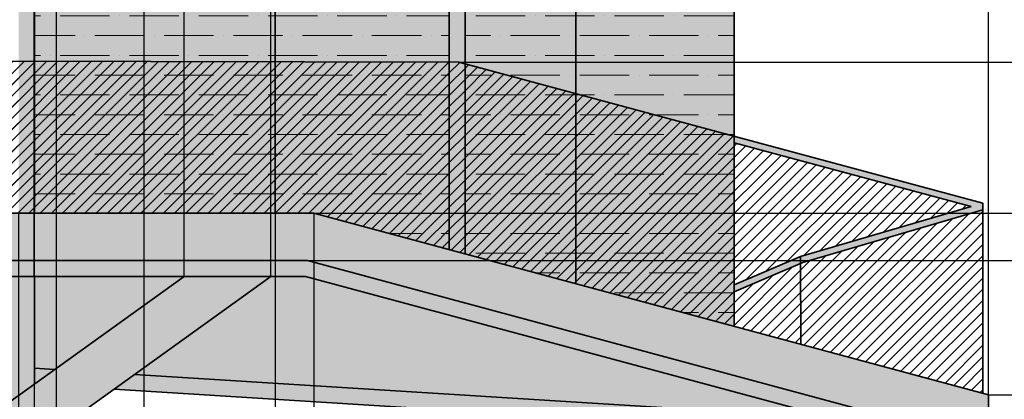
# Model space of a CAD drawing. Units: millimetres. Extents: x -504 to 6314, y 1290 to 4335.
# Tile 7 of 9: x 3796 to 5350, y 2332 to 2932. Entities that reach past the tile are written whole.
import ezdxf

# ---------------------------------------------------------------- set-up
doc = ezdxf.new("R2010")
doc.units = ezdxf.units.MM
doc.header["$MEASUREMENT"] = 0
for name, color, linetype, lineweight in [('A-ANNO-DIMS', 2, 'Continuous', 18), ('A-ELEV', 7, 'Continuous', 35), ('A-ELEV-PATT', 8, 'Continuous', 13)]:
    doc.layers.add(name, color=color, linetype=linetype, lineweight=lineweight)
doc.styles.get("Standard").update_dxf_attribs({"font": 'arial.ttf'})
doc.dimstyles.get("Standard").update_dxf_attribs({"dimtxt": 150, "dimasz": 100, "dimexe": 0.18, "dimexo": 0.0625, "dimgap": 0.09, "dimtad": 0, "dimtih": 1, "dimtoh": 1, "dimdec": 0, "dimzin": 0, "dimdsep": 46, "dimtxsty": 'Standard', "dimcen": 0.09, "dimadec": 0, "dimazin": 0, "dimtfac": 1, "dimtdec": 0, "dimtofl": 0, "dimtmove": 0, "dimatfit": 3, "dimfxl": 1, "dimtolj": 1, "dimtzin": 0, "dimarcsym": 0})
pattern_1 = [(50, (0, 0), (71.726, -6.2752), [7.5, -82.5]), (355, (0, 0), (-13.8751, 75.2192), [6, -66]), (100.4514, (5.98, -0.52), (57.8509, 68.944), [6.374, -70.1142]), (46.1842, (0, 20), (106.7241, -16.5519), [11.25, -123.75]), (96.6356, (8.89, 18.62), (93.4662, 97.4119), [9.561, -105.1714]), (351.1842, (0, 20), (93.4662, 97.4119), [9, -99]), (21, (10, 15), (59.6907, -40.2619), [7.5, -82.5]), (326, (10, 15), (24.3315, 72.515), [6, -66]), (71.4514, (14.974, 11.645), (84.0222, 32.2531), [6.374, -70.1142]), (37.5, (0, 0), (1.21599, 33.28939), [0, -65.2, 0, -67, 0, -66.25]), (7.5, (0, 0), (26.30695, 39.44117), [0, -38.2, 0, -63.7, 0, -25.25]), (327.5, (-22.3, 0), (53.38224, -2.25549), [0, -25, 0, -78, 0, -103.5]), (317.5, (-32.3, 0), (58.3186, 10.0105), [0, -32.5, 0, -51.8, 0, -73.5])]

# ---------------------------------------------------------------- blocks, each defined once
blk = doc.blocks.new('*D5')
at = {"layer": 'A-ANNO-DIMS', "color": 0, "lineweight": -2, "transparency": 16777216}
for p, q in [((4260.1, 2625.8), (5589, 2625.8)), ((5588.8, 2525.8), (5588.8, 2215.7)), ((5588.8, 1752.1), (5588.8, 2062.2)), ((72.9, 1652.1), (5589, 1652.1))]:
    blk.add_line(p, q, dxfattribs=at)
at = {"layer": 'A-ANNO-DIMS', "color": 0, "transparency": 16777216}
for points in [[(5572.1, 2525.8), (5605.5, 2525.8), (5588.8, 2625.8)], [(5572.1, 1752.1), (5605.5, 1752.1), (5588.8, 1652.1)]]:
    blk.add_solid(points, dxfattribs=at)
at = {"layer": 'Defpoints', "color": 0, "transparency": 16777216}
for p in [(4260, 2625.8), (5588.8, 2625.8), (72.8, 1652.1)]:
    blk.add_point(p, dxfattribs=at)
at = {"layer": 'A-ANNO-DIMS', "color": 0, "transparency": 16777216, "insert": (5588.8, 2138.9), "char_height": 150, "attachment_point": 5}
blk.add_mtext('\\A1;973.6', dxfattribs=at)
blk = doc.blocks.new('*D27')
at = {"layer": 'A-ANNO-DIMS', "color": 0, "lineweight": -2, "transparency": 16777216}
for p, q in [((5588.8, 3138.9), (5588.8, 3238.9)), ((5588.8, 3238.9), (5688.8, 3238.9)), ((5081.2, 3138.9), (5589, 3138.9)), ((5588.8, 2964.4), (5588.8, 3038.9)), ((4489, 2864.4), (5589, 2864.4))]:
    blk.add_line(p, q, dxfattribs=at)
at = {"layer": 'A-ANNO-DIMS', "color": 0, "transparency": 16777216}
for points in [[(5572.1, 3038.9), (5605.5, 3038.9), (5588.8, 3138.9)], [(5572.1, 2964.4), (5605.5, 2964.4), (5588.8, 2864.4)]]:
    blk.add_solid(points, dxfattribs=at)
at = {"layer": 'Defpoints', "color": 0, "transparency": 16777216}
for p in [(5081.2, 3138.9), (5588.8, 3138.9), (4489, 2864.4)]:
    blk.add_point(p, dxfattribs=at)
at = {"layer": 'A-ANNO-DIMS', "color": 0, "transparency": 16777216, "insert": (6001.2, 3238.9), "char_height": 150, "attachment_point": 5}
blk.add_mtext('\\A1;274.54', dxfattribs=at)
blk = doc.blocks.new('*D29')
at = {"layer": 'A-ANNO-DIMS', "color": 0, "lineweight": -2, "transparency": 16777216}
for p, q in [((5588.8, 2864.4), (5588.8, 2964.4)), ((5588.8, 2964.4), (5688.8, 2964.4)), ((4489, 2864.4), (5589, 2864.4)), ((5588.8, 2725.8), (5588.8, 2764.4)), ((4260.1, 2625.8), (5589, 2625.8))]:
    blk.add_line(p, q, dxfattribs=at)
at = {"layer": 'A-ANNO-DIMS', "color": 0, "transparency": 16777216}
for points in [[(5572.1, 2764.4), (5605.5, 2764.4), (5588.8, 2864.4)], [(5572.1, 2725.8), (5605.5, 2725.8), (5588.8, 2625.8)]]:
    blk.add_solid(points, dxfattribs=at)
at = {"layer": 'Defpoints', "color": 0, "transparency": 16777216}
for p in [(4489, 2864.4), (5588.8, 2864.4), (4260, 2625.8)]:
    blk.add_point(p, dxfattribs=at)
at = {"layer": 'A-ANNO-DIMS', "color": 0, "transparency": 16777216, "insert": (6002.1, 2964.4), "char_height": 150, "attachment_point": 5}
blk.add_mtext('\\A1;238.65', dxfattribs=at)
blk = doc.blocks.new('*D30')
at = {"layer": 'A-ANNO-DIMS', "color": 0, "lineweight": -2, "transparency": 16777216}
for p, q in [((5588.8, 2725.8), (5588.8, 2825.8)), ((5588.8, 2825.8), (5688.8, 2825.8)), ((4260.1, 2625.8), (5589, 2625.8)), ((4250.2, 2550.8), (5589, 2550.8)), ((5588.8, 2450.8), (5588.8, 2350.8))]:
    blk.add_line(p, q, dxfattribs=at)
at = {"layer": 'A-ANNO-DIMS', "color": 0, "transparency": 16777216}
for points in [[(5572.1, 2725.8), (5605.5, 2725.8), (5588.8, 2625.8)], [(5572.1, 2450.8), (5605.5, 2450.8), (5588.8, 2550.8)]]:
    blk.add_solid(points, dxfattribs=at)
at = {"layer": 'Defpoints', "color": 0, "transparency": 16777216}
for p in [(4260, 2625.8), (5588.8, 2625.8), (4250.1, 2550.8)]:
    blk.add_point(p, dxfattribs=at)
at = {"layer": 'A-ANNO-DIMS', "color": 0, "transparency": 16777216, "insert": (5796.3, 2825.8), "char_height": 150, "attachment_point": 5}
blk.add_mtext('\\A1;75', dxfattribs=at)
blk = doc.blocks.new('*D38')
at = {"layer": 'A-ANNO-DIMS', "color": 0, "lineweight": -2, "transparency": 16777216}
for p, q in [((2963.6, 2625.7), (2963.6, 1387.9)), ((3407.8, 2625.7), (3407.8, 1387.9)), ((3063.6, 1388.1), (3307.8, 1388.1)), ((3407.8, 1388.1), (3507.8, 1388.1))]:
    blk.add_line(p, q, dxfattribs=at)
at = {"layer": 'A-ANNO-DIMS', "color": 0, "transparency": 16777216}
for points in [[(3063.6, 1404.8), (3063.6, 1371.5), (2963.6, 1388.1)], [(3307.8, 1404.8), (3307.8, 1371.5), (3407.8, 1388.1)]]:
    blk.add_solid(points, dxfattribs=at)
at = {"layer": 'Defpoints', "color": 0, "transparency": 16777216}
for p in [(2963.6, 2625.8), (3407.8, 2625.8), (3407.8, 1388.1)]:
    blk.add_point(p, dxfattribs=at)
at = {"layer": 'A-ANNO-DIMS', "color": 0, "transparency": 16777216, "insert": (3763.2, 1388.1), "char_height": 150, "attachment_point": 5}
blk.add_mtext('\\A1;444.2', dxfattribs=at)
blk = doc.blocks.new('*D39')
at = {"layer": 'A-ANNO-DIMS', "color": 0, "lineweight": -2, "transparency": 16777216}
for p, q in [((3407.8, 2625.7), (3407.8, 1387.9)), ((3768.6, 2625.7), (3768.6, 1387.9)), ((3507.8, 1388.1), (3668.6, 1388.1)), ((3768.6, 1388.1), (3868.6, 1388.1))]:
    blk.add_line(p, q, dxfattribs=at)
at = {"layer": 'A-ANNO-DIMS', "color": 0, "transparency": 16777216}
for points in [[(3507.8, 1404.8), (3507.8, 1371.5), (3407.8, 1388.1)], [(3668.6, 1404.8), (3668.6, 1371.5), (3768.6, 1388.1)]]:
    blk.add_solid(points, dxfattribs=at)
at = {"layer": 'Defpoints', "color": 0, "transparency": 16777216}
for p in [(3407.8, 2625.8), (3768.6, 2625.8), (3768.6, 1388.1)]:
    blk.add_point(p, dxfattribs=at)
at = {"layer": 'A-ANNO-DIMS', "color": 0, "transparency": 16777216, "insert": (4179.7, 1388.1), "char_height": 150, "attachment_point": 5}
blk.add_mtext('\\A1;360.84', dxfattribs=at)
blk = doc.blocks.new('*D40')
at = {"layer": 'A-ANNO-DIMS', "color": 0, "lineweight": -2, "transparency": 16777216}
for p, q in [((3768.6, 2625.7), (3768.6, 1387.9)), ((3793.6, 2625.7), (3793.6, 1387.9)), ((3668.6, 1388.1), (3568.6, 1388.1)), ((3893.6, 1388.1), (3993.6, 1388.1))]:
    blk.add_line(p, q, dxfattribs=at)
at = {"layer": 'A-ANNO-DIMS', "color": 0, "transparency": 16777216}
for points in [[(3668.6, 1404.8), (3668.6, 1371.5), (3768.6, 1388.1)], [(3893.6, 1404.8), (3893.6, 1371.5), (3793.6, 1388.1)]]:
    blk.add_solid(points, dxfattribs=at)
at = {"layer": 'Defpoints', "color": 0, "transparency": 16777216}
for p in [(3768.6, 2625.8), (3793.6, 2625.8), (3793.6, 1388.1)]:
    blk.add_point(p, dxfattribs=at)
at = {"layer": 'A-ANNO-DIMS', "color": 0, "transparency": 16777216, "insert": (4103, 1388.1), "char_height": 150, "attachment_point": 5}
blk.add_mtext('\\A1;25', dxfattribs=at)
blk = doc.blocks.new('*D41')
at = {"layer": 'A-ANNO-DIMS', "color": 0, "lineweight": -2, "transparency": 16777216}
for p, q in [((3793.6, 2625.7), (3793.6, 1387.9)), ((3818.6, 2625.7), (3818.6, 1387.9)), ((3693.6, 1388.1), (3593.6, 1388.1)), ((3918.6, 1388.1), (4018.6, 1388.1))]:
    blk.add_line(p, q, dxfattribs=at)
at = {"layer": 'A-ANNO-DIMS', "color": 0, "transparency": 16777216}
for points in [[(3693.6, 1404.8), (3693.6, 1371.5), (3793.6, 1388.1)], [(3918.6, 1404.8), (3918.6, 1371.5), (3818.6, 1388.1)]]:
    blk.add_solid(points, dxfattribs=at)
at = {"layer": 'Defpoints', "color": 0, "transparency": 16777216}
for p in [(3793.6, 2625.8), (3818.6, 2625.8), (3818.6, 1388.1)]:
    blk.add_point(p, dxfattribs=at)
at = {"layer": 'A-ANNO-DIMS', "color": 0, "transparency": 16777216, "insert": (4128, 1388.1), "char_height": 150, "attachment_point": 5}
blk.add_mtext('\\A1;25', dxfattribs=at)
blk = doc.blocks.new('*D42')
at = {"layer": 'A-ANNO-DIMS', "color": 0, "lineweight": -2, "transparency": 16777216}
for p, q in [((3818.6, 2625.7), (3818.6, 1387.9)), ((4198.6, 2625.7), (4198.6, 1387.9)), ((3718.6, 1388.1), (3618.6, 1388.1)), ((4298.6, 1388.1), (4398.6, 1388.1))]:
    blk.add_line(p, q, dxfattribs=at)
at = {"layer": 'A-ANNO-DIMS', "color": 0, "transparency": 16777216}
for points in [[(3718.6, 1404.8), (3718.6, 1371.5), (3818.6, 1388.1)], [(4298.6, 1404.8), (4298.6, 1371.5), (4198.6, 1388.1)]]:
    blk.add_solid(points, dxfattribs=at)
at = {"layer": 'Defpoints', "color": 0, "transparency": 16777216}
for p in [(3818.6, 2625.8), (4198.6, 2625.8), (4198.6, 1388.1)]:
    blk.add_point(p, dxfattribs=at)
at = {"layer": 'A-ANNO-DIMS', "color": 0, "transparency": 16777216, "insert": (4008.6, 1388.1), "char_height": 150, "attachment_point": 5}
blk.add_mtext('\\A1;380', dxfattribs=at)
blk = doc.blocks.new('*D43')
at = {"layer": 'A-ANNO-DIMS', "color": 0, "lineweight": -2, "transparency": 16777216}
for p, q in [((4198.6, 2625.7), (4198.6, 1387.9)), ((4260, 2625.7), (4260, 1387.9)), ((4098.6, 1388.1), (3998.6, 1388.1)), ((4360, 1388.1), (4460, 1388.1))]:
    blk.add_line(p, q, dxfattribs=at)
at = {"layer": 'A-ANNO-DIMS', "color": 0, "transparency": 16777216}
for points in [[(4098.6, 1404.8), (4098.6, 1371.5), (4198.6, 1388.1)], [(4360, 1404.8), (4360, 1371.5), (4260, 1388.1)]]:
    blk.add_solid(points, dxfattribs=at)
at = {"layer": 'Defpoints', "color": 0, "transparency": 16777216}
for p in [(4198.6, 2625.8), (4260, 2625.8), (4260, 1388.1)]:
    blk.add_point(p, dxfattribs=at)
at = {"layer": 'A-ANNO-DIMS', "color": 0, "transparency": 16777216, "insert": (4713.8, 1388.1), "char_height": 150, "attachment_point": 5}
blk.add_mtext('\\A1;61.39', dxfattribs=at)
blk = doc.blocks.new('*D60')
at = {"layer": 'A-ANNO-DIMS', "color": 0, "lineweight": -2, "transparency": 16777216}
for p, q in [((3818.6, 2525.8), (3818.6, 4237)), ((3918.6, 4236.8), (3955.1, 4236.8)), ((4055.1, 2525.8), (4055.1, 4237)), ((4055.1, 4236.8), (4155.1, 4236.8))]:
    blk.add_line(p, q, dxfattribs=at)
at = {"layer": 'A-ANNO-DIMS', "color": 0, "transparency": 16777216}
for points in [[(3918.6, 4253.4), (3918.6, 4220.1), (3818.6, 4236.8)], [(3955.1, 4253.4), (3955.1, 4220.1), (4055.1, 4236.8)]]:
    blk.add_solid(points, dxfattribs=at)
at = {"layer": 'Defpoints', "color": 0, "transparency": 16777216}
for p in [(4055.1, 4236.8), (3818.6, 2525.8), (4055.1, 2525.8)]:
    blk.add_point(p, dxfattribs=at)
at = {"layer": 'A-ANNO-DIMS', "color": 0, "transparency": 16777216, "insert": (4410.2, 4236.8), "char_height": 150, "attachment_point": 5}
blk.add_mtext('\\A1;236.5', dxfattribs=at)
blk = doc.blocks.new('*D61')
at = {"layer": 'A-ANNO-DIMS', "color": 0, "lineweight": -2, "transparency": 16777216}
for p, q in [((3955.1, 4236.8), (3855.1, 4236.8)), ((4055.1, 2525.8), (4055.1, 4237)), ((4192.1, 2525.8), (4192.1, 4237)), ((4292.1, 4236.8), (4392.1, 4236.8))]:
    blk.add_line(p, q, dxfattribs=at)
at = {"layer": 'A-ANNO-DIMS', "color": 0, "transparency": 16777216}
for points in [[(3955.1, 4253.4), (3955.1, 4220.1), (4055.1, 4236.8)], [(4292.1, 4253.4), (4292.1, 4220.1), (4192.1, 4236.8)]]:
    blk.add_solid(points, dxfattribs=at)
at = {"layer": 'Defpoints', "color": 0, "transparency": 16777216}
for p in [(4192.1, 4236.8), (4055.1, 2525.8), (4192.1, 2525.8)]:
    blk.add_point(p, dxfattribs=at)
at = {"layer": 'A-ANNO-DIMS', "color": 0, "transparency": 16777216, "insert": (4550.9, 4236.8), "char_height": 150, "attachment_point": 5}
blk.add_mtext('\\A1;137', dxfattribs=at)
blk = doc.blocks.new('*D62')
at = {"layer": 'A-ANNO-DIMS', "color": 0, "lineweight": -2, "transparency": 16777216}
for p, q in [((4192.1, 2525.8), (4192.1, 4237)), ((4292.1, 4236.8), (4454.1, 4236.8)), ((5224.8, 4236.8), (5062.8, 4236.8)), ((5324.8, 2338.9), (5324.8, 4237))]:
    blk.add_line(p, q, dxfattribs=at)
at = {"layer": 'A-ANNO-DIMS', "color": 0, "transparency": 16777216}
for points in [[(4292.1, 4253.4), (4292.1, 4220.1), (4192.1, 4236.8)], [(5224.8, 4253.4), (5224.8, 4220.1), (5324.8, 4236.8)]]:
    blk.add_solid(points, dxfattribs=at)
at = {"layer": 'Defpoints', "color": 0, "transparency": 16777216}
for p in [(5324.8, 4236.8), (4192.1, 2525.8), (5324.8, 2338.8)]:
    blk.add_point(p, dxfattribs=at)
at = {"layer": 'A-ANNO-DIMS', "color": 0, "transparency": 16777216, "insert": (4758.5, 4236.8), "char_height": 150, "attachment_point": 5}
blk.add_mtext('\\A1;1132.7', dxfattribs=at)
blk = doc.blocks.new('*D65')
at = {"layer": 'A-ANNO-DIMS', "color": 0, "lineweight": -2, "transparency": 16777216}
for p, q in [((5588.8, 2438.8), (5588.8, 2538.8)), ((5588.8, 2538.8), (5688.8, 2538.8)), ((5324.9, 2338.8), (5589, 2338.8)), ((4933.4, 2285.7), (5589, 2285.7)), ((5588.8, 2185.7), (5588.8, 2085.7))]:
    blk.add_line(p, q, dxfattribs=at)
at = {"layer": 'A-ANNO-DIMS', "color": 0, "transparency": 16777216}
for points in [[(5572.1, 2438.8), (5605.5, 2438.8), (5588.8, 2338.8)], [(5572.1, 2185.7), (5605.5, 2185.7), (5588.8, 2285.7)]]:
    blk.add_solid(points, dxfattribs=at)
at = {"layer": 'Defpoints', "color": 0, "transparency": 16777216}
for p in [(5324.8, 2338.8), (5588.8, 2338.8), (4933.3, 2285.7)]:
    blk.add_point(p, dxfattribs=at)
at = {"layer": 'A-ANNO-DIMS', "color": 0, "transparency": 16777216, "insert": (5941.2, 2538.8), "char_height": 150, "attachment_point": 5}
blk.add_mtext('\\A1;53.12', dxfattribs=at)
blk = doc.blocks.new('*D66')
at = {"layer": 'A-ANNO-DIMS', "color": 0, "lineweight": -2, "transparency": 16777216}
for p, q in [((3753.7, 4236.8), (3653.7, 4236.8)), ((3853.7, 1932.9), (3853.7, 4237)), ((3992.1, 1982.9), (3992.1, 4237)), ((4092.1, 4236.8), (4192.1, 4236.8))]:
    blk.add_line(p, q, dxfattribs=at)
at = {"layer": 'A-ANNO-DIMS', "color": 0, "transparency": 16777216}
for points in [[(3753.7, 4253.4), (3753.7, 4220.1), (3853.7, 4236.8)], [(4092.1, 4253.4), (4092.1, 4220.1), (3992.1, 4236.8)]]:
    blk.add_solid(points, dxfattribs=at)
at = {"layer": 'Defpoints', "color": 0, "transparency": 16777216}
for p in [(3992.1, 4236.8), (3992.1, 1982.8), (3853.7, 1932.8)]:
    blk.add_point(p, dxfattribs=at)
at = {"layer": 'A-ANNO-DIMS', "color": 0, "transparency": 16777216, "insert": (4496.6, 4236.8), "char_height": 150, "attachment_point": 5}
blk.add_mtext('\\A1;138.38', dxfattribs=at)

msp = doc.modelspace()

# ---------------------------------------------------------------- hatches: boundary and pattern name
at = {"layer": 'A-ELEV-PATT'}
h = msp.add_hatch(dxfattribs=at)
h.set_pattern_fill('AR-CONC', color=256, scale=10, style=0)
h.set_pattern_definition(pattern_1)
h.paths.add_polyline_path([(4308.57, 3440.687), (3929.687, 3440.687), (3407.797, 3440.687), (1778.718, 3440.687), (1828.718, 3340.687), (3407.797, 3340.687), (3929.687, 3340.687), (4304.463, 3340.687), (5081.168, 3138.941), (5082.876, 3139.564), (5082.876, 3239.564)])
h.paths.add_polyline_path([(4260.021, 2625.758), (3929.687, 2625.758), (3407.797, 2625.758), (2186.182, 2625.758), (2223.682, 2550.758), (3407.797, 2550.758), (3929.687, 2550.758), (4250.093, 2550.758), (5324.792, 2261.16), (5324.792, 2338.836)])
h = msp.add_hatch(color=256, dxfattribs=at)
h.paths.add_polyline_path([(4304.463, 3340.687), (3929.687, 3340.687), (3407.797, 3340.687), (1828.718, 3340.687), (1853.718, 3290.687), (1976.702, 3290.687), (2309.166, 2625.758), (2353.888, 2625.758), (2021.423, 3290.687), (2963.634, 3290.687), (2963.634, 3265.687), (3407.797, 3265.687), (3768.634, 3265.687), (3768.634, 3290.687), (3793.634, 3290.687), (3793.634, 2625.758), (3818.634, 2625.758), (3818.634, 3290.687), (3929.687, 3290.687), (4198.634, 3290.687), (4473.634, 3219.257), (4473.634, 2568.197), (4498.634, 2561.46), (4498.634, 3167.307), (4673.634, 3167.307), (4923.634, 3102.371), (4923.634, 3081.487), (5081.168, 3138.941)])
h.paths.add_polyline_path([(3768.634, 3240.687), (3407.797, 3240.687), (2963.634, 3240.687), (2963.634, 3290.687), (2913.634, 3290.687), (2913.634, 2625.758), (2963.634, 2625.758), (2963.634, 3215.687), (3407.797, 3215.687), (3768.634, 3215.687)], flags=17)
h = msp.add_hatch(color=256, dxfattribs=at)
h.paths.add_polyline_path([(2888.634, 3290.687), (2021.423, 3290.687), (2353.888, 2625.758), (2888.634, 2625.758)])
h.paths.add_polyline_path([(4198.634, 3290.687), (3929.687, 3290.687), (3818.634, 3290.687), (3818.634, 2625.758), (3929.687, 2625.758), (4198.634, 2625.758)])
h.paths.add_polyline_path([(4473.634, 3219.257), (4198.634, 3290.687), (4198.634, 2625.758), (4260.021, 2625.758), (4473.634, 2568.197)])
h.paths.add_polyline_path([(4673.634, 3167.307), (4498.634, 3167.307), (4498.634, 2561.46), (4673.634, 2514.303)])
h.paths.add_polyline_path([(4923.634, 3102.371), (4673.634, 3167.307), (4673.634, 2514.303), (4923.634, 2446.935)])
h = msp.add_hatch(dxfattribs=at)
h.set_pattern_fill('ANSI36', color=256, scale=250, angle=135, style=0)
h.paths.add_polyline_path([(2888.634, 3290.687), (2021.423, 3290.687), (2231.996, 2869.543), (2888.634, 2868.048)])
h.paths.add_polyline_path([(4198.634, 3290.687), (3929.687, 3290.687), (3818.634, 3290.687), (3818.634, 2865.931), (4198.634, 2865.066)])
h.paths.add_polyline_path([(4473.634, 3219.257), (4198.634, 3290.687), (4198.634, 2865.066), (4473.634, 2864.44)])
h.paths.add_polyline_path([(4923.634, 3102.371), (4673.634, 3167.307), (4673.634, 2814.647), (4923.634, 2747.28)])
h.paths.add_polyline_path([(4673.634, 3167.307), (4498.634, 3167.307), (4498.634, 2861.804), (4673.634, 2814.647)])
h.paths.add_polyline_path([(4673.634, 2814.647), (4498.634, 2861.804), (4498.634, 2561.46), (4673.634, 2514.303)])
h.paths.add_polyline_path([(4923.634, 2747.28), (4673.634, 2814.647), (4673.634, 2514.303), (4923.634, 2446.935)])
h.paths.add_polyline_path([(4473.634, 2864.44), (4198.634, 2865.066), (4198.634, 2625.758), (4260.021, 2625.758), (4473.634, 2568.197)])
h.paths.add_polyline_path([(4198.634, 2865.066), (3818.634, 2865.931), (3818.634, 2625.758), (3929.687, 2625.758), (4198.634, 2625.758)])
h.paths.add_polyline_path([(2888.634, 2868.048), (2231.996, 2869.543), (2353.888, 2625.758), (2888.634, 2625.758)])
h = msp.add_hatch(dxfattribs=at)
h.set_pattern_fill('ANSI31', color=256, scale=100, style=0)
h.paths.add_polyline_path([(2888.634, 2868.048), (2231.996, 2869.543), (2353.888, 2625.758), (2888.634, 2625.758)])
h.paths.add_polyline_path([(2913.634, 2867.991), (2888.634, 2868.048), (2888.634, 2625.758), (2913.634, 2625.758)])
h.paths.add_polyline_path([(2963.634, 2867.877), (2913.634, 2867.991), (2913.634, 2625.758), (2963.634, 2625.758)])
h.paths.add_polyline_path([(2963.634, 2852.466), (2963.634, 2625.758), (3076.987, 2625.758)], flags=17)
h.paths.add_polyline_path([(3418.634, 2866.842), (2963.634, 2867.877), (2963.634, 2852.466), (3076.987, 2625.758), (3407.797, 2625.758), (3418.634, 2625.758)])
h.paths.add_polyline_path([(3793.634, 2865.988), (3768.634, 2866.045), (3768.634, 2625.758), (3793.634, 2625.758)])
h.paths.add_polyline_path([(3818.634, 2865.931), (3793.634, 2865.988), (3793.634, 2625.758), (3818.634, 2625.758)])
h.paths.add_polyline_path([(4198.634, 2865.066), (3818.634, 2865.931), (3818.634, 2625.758), (3929.687, 2625.758), (4198.634, 2625.758)])
h.paths.add_polyline_path([(4473.634, 2864.44), (4198.634, 2865.066), (4198.634, 2625.758), (4260.021, 2625.758), (4473.634, 2568.197)])
h.paths.add_polyline_path([(4673.634, 2814.647), (4498.634, 2861.804), (4498.634, 2561.46), (4673.634, 2514.303)])
h.paths.add_polyline_path([(4923.634, 2747.28), (4673.634, 2814.647), (4673.634, 2514.303), (4923.634, 2446.935)])
h.paths.add_polyline_path([(5297.748, 2636.111), (4923.634, 2736.923), (4923.634, 2512.3), (5028.262, 2557.166)])
h.paths.add_polyline_path([(5028.284, 2546.295), (4923.634, 2501.42), (4923.634, 2446.935), (5028.548, 2418.664)])
h.paths.add_polyline_path([(5316.163, 2631.085), (5031.65, 2547.739), (5028.284, 2546.295), (5028.548, 2418.664), (5316.163, 2341.161)])
h = msp.add_hatch(dxfattribs=at)
h.set_pattern_fill('ANSI31', color=256, scale=100, style=0)
h.paths.add_polyline_path([(3793.634, 2865.988), (3768.634, 2866.045), (3768.634, 2625.758), (3793.634, 2625.758)])
h.paths.add_polyline_path([(4498.634, 2861.804), (4488.98, 2864.406), (4473.634, 2864.44), (4473.634, 2568.197), (4498.634, 2561.46)])
h = msp.add_hatch(color=256, dxfattribs=at)
h.paths.add_polyline_path([(5316.163, 2641.506), (4923.634, 2747.28), (4923.634, 2736.923), (5297.748, 2636.111), (5028.262, 2557.166), (5028.284, 2546.295), (5031.65, 2547.739), (5316.163, 2631.085)])
h.paths.add_polyline_path([(5028.262, 2557.166), (4923.634, 2512.3), (4923.634, 2501.42), (5028.284, 2546.295)])
for points in [[(5324.792, 2261.16), (5324.792, 2338.836), (4260.021, 2625.758), (3929.687, 2625.758), (3407.797, 2625.758), (2186.182, 2625.758), (2223.682, 2550.758), (3407.797, 2550.758), (3929.687, 2550.758), (4250.093, 2550.758)], [(4250.093, 2550.758), (3929.687, 2550.758), (3407.797, 2550.758), (2223.682, 2550.758), (2236.182, 2525.758), (3407.797, 2525.758), (3929.687, 2525.758), (4246.784, 2525.758), (5078.405, 2301.662), (3976.669, 2370.761), (3944.641, 2347.72), (5324.792, 2261.16)], [(3850.662, 2378.664), (3818.634, 2380.672), (3818.634, 2355.623)]]:
    msp.add_hatch(color=256, dxfattribs=at).paths.add_polyline_path(points)
h = msp.add_hatch(dxfattribs=at)
h.set_pattern_fill('AR-CONC', color=256, scale=10, style=0)
h.set_pattern_definition(pattern_1)
h.paths.add_polyline_path([(4260.021, 2625.758), (3929.687, 2625.758), (3407.797, 2625.758), (2186.182, 2625.758), (2223.682, 2550.758), (3407.797, 2550.758), (3929.687, 2550.758), (4250.093, 2550.758), (5324.792, 2261.16), (5324.792, 2338.836)])
h = msp.add_hatch(color=256, dxfattribs=at)
h.paths.add_polyline_path([(4192.131, 2525.758), (4055.138, 2525.758), (2840.705, 1652.125), (2977.698, 1652.125)])
h.paths.add_polyline_path([(4718.141, 2299.208), (4608.219, 2306.102), (3872.15, 1776.591), (3922.329, 1726.72)])
h = msp.add_hatch(color=256, dxfattribs=at)
h.paths.add_polyline_path([(3447.81, 1943.758), (3768.634, 1943.758), (3768.634, 1968.758), (3447.81, 1968.758), (3447.81, 1990.312), (3383.096, 1943.758), (3397.81, 1943.758), (3397.81, 1702.125), (3076.987, 1702.125), (3076.987, 1652.125), (3818.634, 1652.125), (3818.634, 2257.074), (3768.634, 2221.105), (3768.634, 1702.125), (3447.81, 1702.125)])
h.paths.add_polyline_path([(3650.62, 2234.758), (3447.81, 2234.758), (3447.81, 2475.758), (3768.634, 2475.758), (3768.634, 2319.654), (3818.634, 2355.623), (3818.634, 2525.758), (3407.797, 2525.758), (3076.987, 2525.758), (3076.987, 2475.758), (3397.81, 2475.758), (3397.81, 2234.758), (3076.987, 2234.758), (3076.987, 2209.758), (3397.81, 2209.758), (3397.81, 2052.893), (3447.81, 2088.862), (3447.81, 2209.758), (3615.868, 2209.758)])
h.paths.add_polyline_path([(3280.855, 1968.758), (3076.987, 1968.758), (3076.987, 1943.758), (3246.103, 1943.758)], flags=17)
h.paths.add_polyline_path([(3768.634, 2221.105), (3752.861, 2209.758), (3768.634, 2209.758)], flags=17)
h = msp.add_hatch(color=256, dxfattribs=at)
h.set_gradient(color1=(99, 100, 102), color2=(0, 0, 0), name='CYLINDER')
h.paths.add_polyline_path([(5078.405, 2301.662), (4246.784, 2525.758), (4192.131, 2525.758), (3976.669, 2370.761)])
h.paths.add_polyline_path([(4055.138, 2525.758), (3929.687, 2525.758), (3818.634, 2525.758), (3818.634, 2380.672), (3850.662, 2378.664)])

# ---------------------------------------------------------------- linework, layer by layer
at = {"layer": 'A-ELEV'}
for p, q in [((3818.634, 3290.687), (3818.634, 2625.758)), ((4198.634, 3290.687), (4198.634, 2625.758)), ((4473.634, 3219.257), (4473.634, 2568.197)), ((4498.634, 3167.307), (4498.634, 2561.46)), ((4673.634, 3167.307), (4673.634, 2514.303)), ((4923.634, 3102.371), (4923.634, 2446.935)), ((2231.996, 2869.543), (4488.98, 2864.406)), ((4488.98, 2864.406), (5316.163, 2641.506)), ((4923.634, 2736.923), (5297.748, 2636.111)), ((5297.748, 2636.111), (5028.262, 2557.166)), ((5316.163, 2631.085), (5031.65, 2547.739)), ((5316.163, 2341.161), (5316.163, 2641.506)), ((3407.797, 2625.758), (3929.687, 2625.758)), ((3929.687, 2625.758), (4260.021, 2625.758)), ((4260.021, 2625.758), (5324.792, 2338.836)), ((3407.797, 2550.758), (3929.687, 2550.758)), ((3929.687, 2550.758), (4250.093, 2550.758)), ((4250.093, 2550.758), (5324.792, 2261.16)), ((5028.262, 2557.166), (4923.634, 2512.3)), ((5028.262, 2557.166), (5028.548, 2418.664)), ((5031.65, 2547.739), (4923.634, 2501.42)), ((2840.705, 1652.125), (4055.138, 2525.758)), ((2977.698, 1652.125), (4192.131, 2525.758)), ((3407.797, 2525.758), (3929.687, 2525.758)), ((3818.634, 2355.623), (3818.634, 2525.758)), ((3929.687, 2525.758), (4246.784, 2525.758)), ((4246.784, 2525.758), (5078.405, 2301.662)), ((3850.662, 2378.664), (3818.634, 2380.672)), ((5078.405, 2301.662), (3976.669, 2370.761)), ((5324.792, 2261.16), (3944.641, 2347.72)), ((5324.792, 2261.16), (5324.792, 2338.836))]:
    msp.add_line(p, q, dxfattribs=at)

# ---------------------------------------------------------------- dimensions: what is measured, and where the dimension line sits
at = {"layer": 'A-ANNO-DIMS'}
for base, p1, p2, override, picture, middle in [((3992.087, 4236.781), (3853.708, 1932.831), (3992.087, 1982.831), {"dimdec": 2, "dimlfac": 1, "dimrnd": 0, "dimzin": 0, "dimdsep": 46, "dimlunit": 2}, '*D66', (4496.628, 4236.781)), ((4055.138, 4236.781), (3818.634, 2525.758), (4055.138, 2525.758), {"dimdec": 1, "dimlfac": 1, "dimrnd": 0, "dimzin": 0, "dimdsep": 46, "dimlunit": 2}, '*D60', (4410.156, 4236.781)), ((4192.131, 4236.781), (4055.138, 2525.758), (4192.131, 2525.758), {"dimdec": 0, "dimlfac": 1, "dimrnd": 0, "dimzin": 0, "dimdsep": 46, "dimlunit": 2}, '*D61', (4550.867, 4236.781)), ((5324.792, 4236.781), (4192.131, 2525.758), (5324.792, 2338.836), {"dimdec": 1, "dimlfac": 1, "dimrnd": 0, "dimzin": 0, "dimdsep": 46, "dimlunit": 2}, '*D62', (4758.461, 4236.781)), ((3407.797, 1388.125), (2963.634, 2625.758), (3407.797, 2625.758), {"dimdec": 1, "dimlfac": 1, "dimrnd": 0, "dimzin": 0, "dimdsep": 46, "dimlunit": 2}, '*D38', (3763.224, 1388.125)), ((3768.634, 1388.125), (3407.797, 2625.758), (3768.634, 2625.758), {"dimdec": 2, "dimlfac": 1, "dimrnd": 0, "dimzin": 0, "dimdsep": 46, "dimlunit": 2}, '*D39', (4179.723, 1388.125)), ((3793.634, 1388.125), (3768.634, 2625.758), (3793.634, 2625.758), {"dimdec": 0, "dimlfac": 1, "dimrnd": 0, "dimzin": 0, "dimdsep": 46, "dimlunit": 2}, '*D40', (4103.001, 1388.125)), ((3818.634, 1388.125), (3793.634, 2625.758), (3818.634, 2625.758), {"dimdec": 0, "dimlfac": 1, "dimrnd": 0, "dimzin": 0, "dimdsep": 46, "dimlunit": 2}, '*D41', (4128.001, 1388.125)), ((4198.634, 1388.125), (3818.634, 2625.758), (4198.634, 2625.758), {"dimdec": 0, "dimlfac": 1, "dimrnd": 0, "dimzin": 0, "dimdsep": 46, "dimlunit": 2}, '*D42', (4008.634, 1388.125)), ((4260.021, 1388.125), (4198.634, 2625.758), (4260.021, 2625.758), {"dimdec": 2, "dimlfac": 1, "dimrnd": 0, "dimzin": 0, "dimdsep": 46, "dimlunit": 2}, '*D43', (4713.761, 1388.125))]:
    dim = msp.add_linear_dim(base=base, p1=p1, p2=p2, dimstyle='Standard', override=override, dxfattribs=at)
    dim.commit()
    dim.dimension.update_dxf_attribs({"geometry": picture, "text_midpoint": middle})
for base, p1, p2, override, picture, middle in [((5588.7921, 3138.9408), (4488.9803, 2864.4056), (5081.1676, 3138.9408), {"dimdec": 2, "dimlfac": 1, "dimrnd": 0, "dimzin": 0, "dimdsep": 46, "dimlunit": 2}, '*D27', (6001.2116, 3238.9408)), ((5588.792, 2864.406), (4260.021, 2625.758), (4488.98, 2864.406), {"dimdec": 2, "dimlfac": 1, "dimrnd": 0, "dimzin": 0, "dimdsep": 46, "dimlunit": 2}, '*D29', (6002.081, 2964.406)), ((5588.792, 2625.758), (4250.093, 2550.758), (4260.021, 2625.758), {"dimdec": 0, "dimlfac": 1, "dimrnd": 0, "dimzin": 0, "dimdsep": 46, "dimlunit": 2}, '*D30', (5796.266, 2825.758)), ((5588.792, 2338.836), (4933.327, 2285.712), (5324.792, 2338.836), {"dimdec": 2, "dimlfac": 1, "dimrnd": 0, "dimzin": 0, "dimdsep": 46, "dimlunit": 2}, '*D65', (5941.201, 2538.836)), ((5588.792, 2625.758), (72.835, 1652.125), (4260.021, 2625.758), {"dimdec": 1, "dimlfac": 1, "dimrnd": 0, "dimzin": 0, "dimdsep": 46, "dimlunit": 2}, '*D5', (5588.792, 2138.941))]:
    dim = msp.add_linear_dim(base=base, p1=p1, p2=p2, angle=90, dimstyle='Standard', override=override, dxfattribs=at)
    dim.commit()
    dim.dimension.update_dxf_attribs({"geometry": picture, "text_midpoint": middle})

doc.saveas('drawing.dxf')
